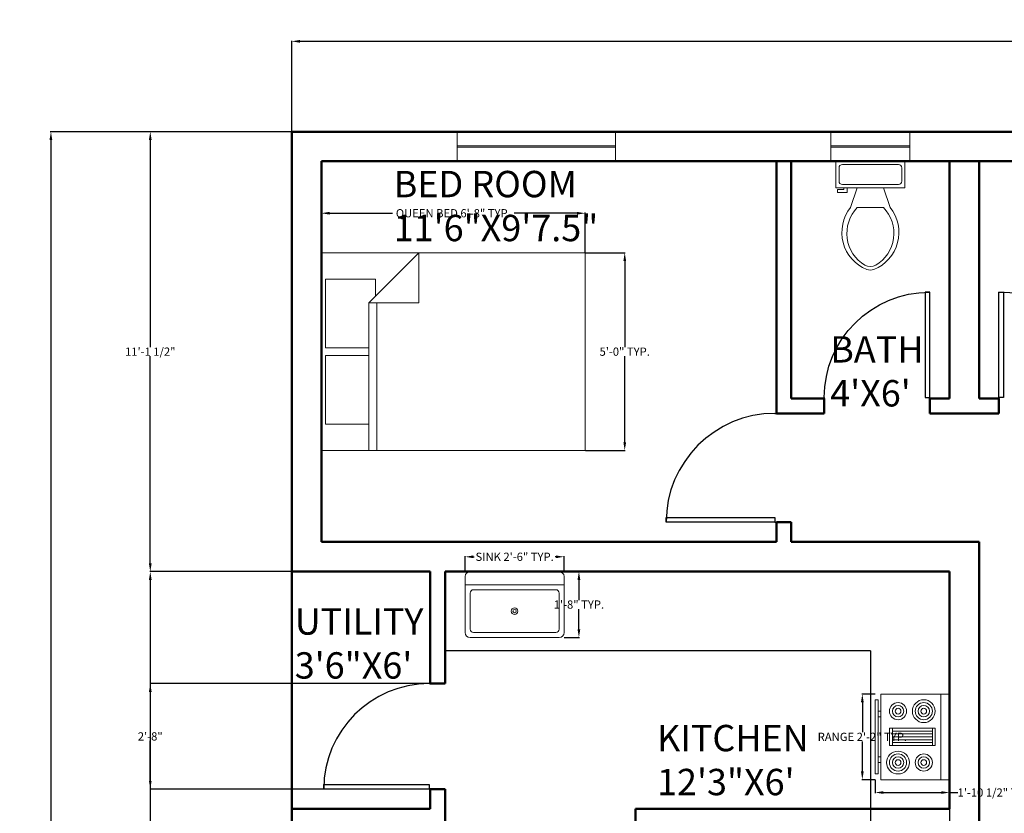
# Model space of a CAD drawing. Units: inches. Extents: x -46 to 565, y -56 to 809.
# Tile 4 of 6: x -46 to 252, y 557 to 798. Entities that reach past the tile are written whole.
import ezdxf

# ---------------------------------------------------------------- set-up
doc = ezdxf.new("R2010")
doc.units = ezdxf.units.IN
doc.header["$MEASUREMENT"] = 0
for name, color, linetype, lineweight in [('A-ANNO-DIMS', 2, 'Continuous', 18), ('A-AREA-IDEN', 241, 'Continuous', 18), ('A-FLOR-CASE', 8, 'Continuous', 25), ('A-FLOR-FIXT', 131, 'Continuous', 18), ('A-FURN', 131, 'Continuous', 18), ('DOOR', 210, 'Continuous', 25), ('EQUIPMENT', 131, 'Continuous', 18), ('WALL', 10, 'Continuous', 50), ('WINDOW', 170, 'Continuous', 18)]:
    doc.layers.add(name, color=color, linetype=linetype, lineweight=lineweight)
doc.styles.get("Standard").update_dxf_attribs({"font": 'arial.ttf'})
doc.dimstyles.get("Standard").update_dxf_attribs({"dimtxt": 2.5, "dimasz": 2.5, "dimexe": 0.18, "dimexo": 0.0625, "dimgap": 0.09, "dimtad": 0, "dimtih": 1, "dimtoh": 1, "dimzin": 0, "dimdsep": 46, "dimlunit": 3, "dimtxsty": 'Standard', "dimcen": 0.09, "dimadec": 0, "dimazin": 0, "dimtfac": 1, "dimtofl": 0, "dimtmove": 0, "dimatfit": 3, "dimfxl": 1, "dimtolj": 1, "dimtzin": 0, "dimarcsym": 0})

# ---------------------------------------------------------------- blocks, each defined once
blk = doc.blocks.new('*U2')
for p, q in [((0, 0), (0, -6)), ((40, 0), (40, -6))]:
    blk.add_line(p, q)
blk.add_lwpolyline([(0, 0), (0, 40), (1.75, 40), (1.75, 0)], close=True)
blk.add_arc((0, 0), 40, 0, 90)
blk = doc.blocks.new('Sink-single - 30 in top')
blk.add_line((-15, -3.999996), (15, -3.999996))
for points in [[(-13.5, 0), (13.5, 0)], [(-15, -18.499996), (-15, -1.5)], [(15, -1.5), (15, -18.499996)], [(-12.5, -5.499996), (12.5, -5.499996)], [(-13.5, -17.499996), (-13.5, -6.499996)], [(13.5, -6.499996), (13.5, -17.499996)], [(13.5, -19.999996), (-13.5, -19.999996)], [(12.5, -18.499996), (-12.5, -18.499996)]]:
    blk.add_lwpolyline(points)
for radius in [1, 0.5]:
    blk.add_circle((0, -11.999996), radius)
for centre, radius, start, end in [((-13.5, -1.5), 1.5, 90, 180), ((13.5, -1.5), 1.5, 0, 90), ((-12.5, -6.499996), 1, 90, 180), ((12.5, -6.499996), 1, 0, 90), ((-12.5, -17.499996), 1, 180, 270), ((12.5, -17.499996), 1, 270, 0), ((-13.5, -18.499996), 1.5, 180, 270), ((13.5, -18.499996), 1.5, 270, 0)]:
    blk.add_arc(centre, radius, start, end)
blk = doc.blocks.new('Bed - Queen')
for p, q in [((0, -80.00003), (0, 0)), ((0, 0), (59.99999, 0)), ((59.99999, 0), (59.99999, -80.00003)), ((7.99999, -1.2), (28.79998, -1.2)), ((7.99999, -14.4), (7.99999, -1.2)), ((28.79998, -1.2), (28.79998, -14.4)), ((31.19999, -1.2), (51.99999, -1.2)), ((31.19999, -14.4), (31.19999, -1.2)), ((51.99999, -1.2), (51.99999, -16.4)), ((0, -14.4), (44.8, -14.4)), ((59.99999, -29.6), (44.8, -14.4)), ((44.8, -14.4), (44.8, -29.6)), ((44.8, -16.8), (0, -16.8)), ((51.99999, -16.4), (46.79936, -16.4)), ((44.8, -29.6), (59.99999, -29.6)), ((59.99999, -80.00003), (0, -80.00003))]:
    blk.add_line(p, q)
blk = doc.blocks.new('Toilet - top')
for p, q in [((9.5, -6), (9.5, -2)), ((-10, -8.5), (-8, -8.5)), ((-10, -9.5), (-10, -8.5)), ((-8, -8.5), (-8, -8)), ((-7, -8), (-7, -9.5)), ((-4, -8), (-6, -14)), ((4, -8), (6, -14)), ((-7, -9.5), (-10, -9.5)), ((4, -14), (-4, -14))]:
    blk.add_line(p, q)
blk.add_lwpolyline([(10.5, -8), (10.5, 0), (-10.5, 0), (-10.5, -8)], close=True)
for points in [[(-9.5, -2), (-9.5, -6)], [(8.5, -1), (-8.5, -1)], [(-8.5, -7), (8.5, -7)]]:
    blk.add_lwpolyline(points)
for centre, radius, start, end in [((-8.62, -1.88), 0.884, 81.8699, 188.1301), ((8.62, -1.88), 0.884, 351.8699, 98.1301), ((-8.62, -6.12), 0.884, 171.8699, 278.1301), ((8.62, -6.12), 0.884, 261.8699, 8.1301), ((3.52, -21.58), 12.17, 141.4691, 247.9714), ((4.2, -21.82), 11.33, 136.3677, 238.9468), ((-3.52, -21.58), 12.17, 292.0284, 38.5307), ((-4.2, -21.82), 11.33, 301.053, 43.6321), ((0, -27.88), 4, 245.7318, 294.2682), ((0, -29), 4, 254.8605, 285.1395)]:
    blk.add_arc(centre, radius, start, end)
blk = doc.blocks.new('Range-Oven - 30 in top')
for p, q in [((0, -3), (30, -3)), ((12, -6), (18, -6)), ((13, -20), (13, -6)), ((14, -6), (14, -20)), ((15, -20), (15, -6)), ((16, -6), (16, -20)), ((17, -20), (17, -6)), ((18, -20), (12, -20)), ((6, -24), (6, -25)), ((8, -25), (8, -24)), ((22, -25), (22, -24)), ((24, -24), (24, -25))]:
    blk.add_line(p, q)
for points in [[(0, -24), (0, 0), (30, 0), (30, -24)], [(12, -21), (12, -5), (18, -5), (18, -21)], [(2, -26), (2, -25), (28, -25), (28, -26)]]:
    blk.add_lwpolyline(points, close=True)
for centre, radius in [((6, -9), 4), ((6, -9), 3), ((24, -9), 3), ((6, -9), 2), ((6, -9), 1), ((24, -9), 2), ((24, -9), 1), ((6, -18), 3), ((6, -18), 2), ((6, -18), 1), ((24, -18), 4), ((24, -18), 3), ((24, -18), 2), ((24, -18), 1)]:
    blk.add_circle(centre, radius)
blk = doc.blocks.new('*D14')
at = {"layer": 'A-ANNO-DIMS', "color": 0, "lineweight": -2, "transparency": 16777216}
for p, q in [((36.14, 764.26), (36.14, 791.8)), ((38.64, 791.62), (267.37, 791.62)), ((513.64, 791.62), (284.92, 791.62)), ((516.14, 764.26), (516.14, 791.8))]:
    blk.add_line(p, q, dxfattribs=at)
at = {"layer": 'A-ANNO-DIMS', "color": 0, "transparency": 16777216}
for points in [[(38.64, 792.04), (38.64, 791.2), (36.14, 791.62)], [(513.64, 792.04), (513.64, 791.2), (516.14, 791.62)]]:
    blk.add_solid(points, dxfattribs=at)
at = {"layer": 'Defpoints', "color": 0, "transparency": 16777216}
for p in [(516.14, 791.62), (36.14, 764.2), (516.14, 764.2)]:
    blk.add_point(p, dxfattribs=at)
at = {"layer": 'A-ANNO-DIMS', "color": 0, "transparency": 16777216, "insert": (276.14, 791.62), "char_height": 10, "attachment_point": 5}
blk.add_mtext("\\A1;40'", dxfattribs=at)
blk = doc.blocks.new('*D15')
at = {"layer": 'A-ANNO-DIMS', "color": 0, "lineweight": -2, "transparency": 16777216}
for p, q in [((174.08, 764.2), (-37.07, 764.2)), ((-36.89, 761.7), (-36.89, 409.4)), ((-36.89, 46.7), (-36.89, 399)), ((174.08, 44.2), (-37.07, 44.2))]:
    blk.add_line(p, q, dxfattribs=at)
at = {"layer": 'A-ANNO-DIMS', "color": 0, "transparency": 16777216}
for points in [[(-37.31, 761.7), (-36.48, 761.7), (-36.89, 764.2)], [(-37.31, 46.7), (-36.48, 46.7), (-36.89, 44.2)]]:
    blk.add_solid(points, dxfattribs=at)
at = {"layer": 'Defpoints', "color": 0, "transparency": 16777216}
for p in [(-36.89, 764.2), (174.14, 764.2), (174.14, 44.2)]:
    blk.add_point(p, dxfattribs=at)
at = {"layer": 'A-ANNO-DIMS', "color": 0, "transparency": 16777216, "insert": (-36.89, 404.2), "char_height": 10, "attachment_point": 5}
blk.add_mtext("\\A1;60'", dxfattribs=at)
blk = doc.blocks.new('WIN-48IN')
for p, q in [((0, 4.75), (48, 4.75)), ((0, 4.25), (48, 4.25))]:
    blk.add_line(p, q)
blk.add_lwpolyline([(0, 0), (48, 0), (48, 9), (0, 9)], close=True)
blk = doc.blocks.new('WIN-24IN')
for p, q in [((4.25, 24), (4.25, 0)), ((4.75, 24), (4.75, 0))]:
    blk.add_line(p, q)
blk.add_lwpolyline([(0, 24), (0, 0), (9, 0), (9, 24)], close=True)
blk = doc.blocks.new('*D19')
at = {"layer": 'A-ANNO-DIMS', "color": 0, "lineweight": -2, "transparency": 16777216}
for p, q in [((45.14, 727.51), (45.14, 739.63)), ((47.64, 739.45), (66.67, 739.45)), ((122.64, 739.45), (103.62, 739.45)), ((125.14, 727.51), (125.14, 739.63))]:
    blk.add_line(p, q, dxfattribs=at)
at = {"layer": 'A-ANNO-DIMS', "color": 0, "transparency": 16777216}
for points in [[(47.64, 739.87), (47.64, 739.03), (45.14, 739.45)], [(122.64, 739.87), (122.64, 739.03), (125.14, 739.45)]]:
    blk.add_solid(points, dxfattribs=at)
at = {"layer": 'Defpoints', "color": 0, "transparency": 16777216}
for p in [(45.14, 739.45), (45.14, 727.45), (125.14, 727.45)]:
    blk.add_point(p, dxfattribs=at)
at = {"layer": 'A-ANNO-DIMS', "color": 0, "transparency": 16777216, "insert": (85.14, 739.45), "char_height": 2.5, "attachment_point": 5}
blk.add_mtext('\\A1;QUEEN BED 6\'-8" TYP.', dxfattribs=at)
blk = doc.blocks.new('*D20')
at = {"layer": 'A-ANNO-DIMS', "color": 0, "lineweight": -2, "transparency": 16777216}
for p, q in [((125.21, 727.45), (137.32, 727.45)), ((137.14, 724.95), (137.14, 698.82)), ((137.14, 669.95), (137.14, 696.08)), ((125.21, 667.45), (137.32, 667.45))]:
    blk.add_line(p, q, dxfattribs=at)
at = {"layer": 'A-ANNO-DIMS', "color": 0, "transparency": 16777216}
for points in [[(136.73, 724.95), (137.56, 724.95), (137.14, 727.45)], [(136.73, 669.95), (137.56, 669.95), (137.14, 667.45)]]:
    blk.add_solid(points, dxfattribs=at)
at = {"layer": 'Defpoints', "color": 0, "transparency": 16777216}
for p in [(125.14, 727.45), (137.14, 727.45), (125.14, 667.45)]:
    blk.add_point(p, dxfattribs=at)
at = {"layer": 'A-ANNO-DIMS', "color": 0, "transparency": 16777216, "insert": (137.14, 697.45), "char_height": 2.5, "attachment_point": 5}
blk.add_mtext('\\A1;5\'-0" TYP.', dxfattribs=at)
blk = doc.blocks.new('*D31')
at = {"layer": 'A-ANNO-DIMS', "color": 0, "lineweight": -2, "transparency": 16777216}
for p, q in [((88.75, 630.76), (88.75, 635.38)), ((91.25, 635.2), (91.48, 635.2)), ((116.25, 635.2), (116.01, 635.2)), ((118.75, 630.76), (118.75, 635.38))]:
    blk.add_line(p, q, dxfattribs=at)
at = {"layer": 'A-ANNO-DIMS', "color": 0, "transparency": 16777216}
for points in [[(91.25, 635.62), (91.25, 634.78), (88.75, 635.2)], [(116.25, 635.62), (116.25, 634.78), (118.75, 635.2)]]:
    blk.add_solid(points, dxfattribs=at)
at = {"layer": 'Defpoints', "color": 0, "transparency": 16777216}
for p in [(88.75, 635.2), (88.75, 630.7), (118.75, 630.7)]:
    blk.add_point(p, dxfattribs=at)
at = {"layer": 'A-ANNO-DIMS', "color": 0, "transparency": 16777216, "insert": (103.75, 635.2), "char_height": 2.5, "attachment_point": 5}
blk.add_mtext('\\A1;SINK 2\'-6" TYP.', dxfattribs=at)
blk = doc.blocks.new('*D32')
at = {"layer": 'A-ANNO-DIMS', "color": 0, "lineweight": -2, "transparency": 16777216}
for p, q in [((118.81, 630.7), (123.43, 630.7)), ((123.25, 628.2), (123.25, 622.07)), ((123.25, 613.2), (123.25, 619.33)), ((118.81, 610.7), (123.43, 610.7))]:
    blk.add_line(p, q, dxfattribs=at)
at = {"layer": 'A-ANNO-DIMS', "color": 0, "transparency": 16777216}
for points in [[(122.83, 628.2), (123.67, 628.2), (123.25, 630.7)], [(122.83, 613.2), (123.67, 613.2), (123.25, 610.7)]]:
    blk.add_solid(points, dxfattribs=at)
at = {"layer": 'Defpoints', "color": 0, "transparency": 16777216}
for p in [(118.75, 630.7), (123.25, 630.7), (118.75, 610.7)]:
    blk.add_point(p, dxfattribs=at)
at = {"layer": 'A-ANNO-DIMS', "color": 0, "transparency": 16777216, "insert": (123.25, 620.7), "char_height": 2.5, "attachment_point": 5}
blk.add_mtext('\\A1;1\'-8" TYP.', dxfattribs=at)
blk = doc.blocks.new('*D35')
at = {"layer": 'A-ANNO-DIMS', "color": 0, "lineweight": -2, "transparency": 16777216}
for p, q in [((213.05, 593.56), (209.03, 593.56)), ((209.21, 591.06), (209.21, 581.94)), ((209.21, 570.06), (209.21, 579.18)), ((213.05, 567.56), (209.03, 567.56))]:
    blk.add_line(p, q, dxfattribs=at)
at = {"layer": 'A-ANNO-DIMS', "color": 0, "transparency": 16777216}
for points in [[(208.79, 591.06), (209.63, 591.06), (209.21, 593.56)], [(208.79, 570.06), (209.63, 570.06), (209.21, 567.56)]]:
    blk.add_solid(points, dxfattribs=at)
at = {"layer": 'Defpoints', "color": 0, "transparency": 16777216}
for p in [(213.11, 593.56), (209.21, 567.56), (213.11, 567.56)]:
    blk.add_point(p, dxfattribs=at)
at = {"layer": 'A-ANNO-DIMS', "color": 0, "transparency": 16777216, "insert": (209.21, 580.56), "char_height": 2.5, "attachment_point": 5}
blk.add_mtext('\\A1;RANGE 2\'-2" TYP.', dxfattribs=at)
blk = doc.blocks.new('*D36')
at = {"layer": 'A-ANNO-DIMS', "color": 0, "lineweight": -2, "transparency": 16777216}
for p, q in [((213.11, 567.5), (213.11, 563.48)), ((235.64, 567.5), (235.64, 563.48)), ((215.61, 563.66), (233.14, 563.66)), ((235.64, 563.66), (238.14, 563.66))]:
    blk.add_line(p, q, dxfattribs=at)
at = {"layer": 'A-ANNO-DIMS', "color": 0, "transparency": 16777216}
for points in [[(215.61, 564.08), (215.61, 563.24), (213.11, 563.66)], [(233.14, 564.08), (233.14, 563.24), (235.64, 563.66)]]:
    blk.add_solid(points, dxfattribs=at)
at = {"layer": 'Defpoints', "color": 0, "transparency": 16777216}
for p in [(213.11, 567.56), (235.64, 567.56), (235.64, 563.66)]:
    blk.add_point(p, dxfattribs=at)
at = {"layer": 'A-ANNO-DIMS', "color": 0, "transparency": 16777216, "insert": (249.62, 563.66), "char_height": 2.5, "attachment_point": 5}
blk.add_mtext('\\A1;1\'-10 1/2" TYP.', dxfattribs=at)
blk = doc.blocks.new('*D46')
at = {"layer": 'A-ANNO-DIMS', "color": 0, "lineweight": -2, "transparency": 16777216}
for p, q in [((36.08, 630.7), (-6.94, 630.7)), ((-6.76, 628.2), (-6.76, 464.54)), ((-6.76, 298.2), (-6.76, 461.85)), ((45.08, 295.7), (-6.94, 295.7))]:
    blk.add_line(p, q, dxfattribs=at)
at = {"layer": 'A-ANNO-DIMS', "color": 0, "transparency": 16777216}
for points in [[(-7.17, 628.2), (-6.34, 628.2), (-6.76, 630.7)], [(-7.17, 298.2), (-6.34, 298.2), (-6.76, 295.7)]]:
    blk.add_solid(points, dxfattribs=at)
at = {"layer": 'Defpoints', "color": 0, "transparency": 16777216}
for p in [(-6.76, 630.7), (36.14, 630.7), (45.14, 295.7)]:
    blk.add_point(p, dxfattribs=at)
at = {"layer": 'A-ANNO-DIMS', "color": 0, "transparency": 16777216, "insert": (-6.76, 463.2), "char_height": 2.5, "attachment_point": 5}
blk.add_mtext('\\A1;27\'-11"', dxfattribs=at)
blk = doc.blocks.new('*D47')
at = {"layer": 'A-ANNO-DIMS', "color": 0, "lineweight": -2, "transparency": 16777216}
for p, q in [((36.08, 764.2), (-6.94, 764.2)), ((-6.76, 761.7), (-6.76, 698.83)), ((-6.76, 633.2), (-6.76, 696.07)), ((36.08, 630.7), (-6.94, 630.7))]:
    blk.add_line(p, q, dxfattribs=at)
at = {"layer": 'A-ANNO-DIMS', "color": 0, "transparency": 16777216}
for points in [[(-7.17, 761.7), (-6.34, 761.7), (-6.76, 764.2)], [(-7.17, 633.2), (-6.34, 633.2), (-6.76, 630.7)]]:
    blk.add_solid(points, dxfattribs=at)
at = {"layer": 'Defpoints', "color": 0, "transparency": 16777216}
for p in [(-6.76, 764.2), (36.14, 764.2), (36.14, 630.7)]:
    blk.add_point(p, dxfattribs=at)
at = {"layer": 'A-ANNO-DIMS', "color": 0, "transparency": 16777216, "insert": (-6.76, 697.45), "char_height": 2.5, "attachment_point": 5}
blk.add_mtext('\\A1;11\'-1 1/2"', dxfattribs=at)
blk = doc.blocks.new('*D50')
at = {"layer": 'A-ANNO-DIMS', "color": 0, "lineweight": -2, "transparency": 16777216}
for p, q in [((211.64, 558.64), (211.64, 0.22)), ((235.64, 558.64), (235.64, 0.22)), ((214.14, 0.4), (220.21, 0.4)), ((233.14, 0.4), (227.08, 0.4))]:
    blk.add_line(p, q, dxfattribs=at)
at = {"layer": 'A-ANNO-DIMS', "color": 0, "transparency": 16777216}
for points in [[(214.14, 0.82), (214.14, -0.02), (211.64, 0.4)], [(233.14, 0.82), (233.14, -0.02), (235.64, 0.4)]]:
    blk.add_solid(points, dxfattribs=at)
at = {"layer": 'Defpoints', "color": 0, "transparency": 16777216}
for p in [(211.64, 558.7), (235.64, 558.7), (235.64, 0.4)]:
    blk.add_point(p, dxfattribs=at)
at = {"layer": 'A-ANNO-DIMS', "color": 0, "transparency": 16777216, "insert": (223.64, 0.4), "char_height": 2.5, "attachment_point": 5}
blk.add_mtext('\\A1;2\'-0"', dxfattribs=at)
blk = doc.blocks.new('*D52')
at = {"layer": 'A-ANNO-DIMS', "color": 0, "lineweight": -2, "transparency": 16777216}
for p, q in [((78.08, 596.7), (-6.94, 596.7)), ((-6.76, 594.2), (-6.76, 582.07)), ((-6.76, 567.2), (-6.76, 579.33)), ((78.08, 564.7), (-6.94, 564.7))]:
    blk.add_line(p, q, dxfattribs=at)
at = {"layer": 'A-ANNO-DIMS', "color": 0, "transparency": 16777216}
for points in [[(-7.17, 594.2), (-6.34, 594.2), (-6.76, 596.7)], [(-7.17, 567.2), (-6.34, 567.2), (-6.76, 564.7)]]:
    blk.add_solid(points, dxfattribs=at)
at = {"layer": 'Defpoints', "color": 0, "transparency": 16777216}
for p in [(-6.76, 596.7), (78.14, 596.7), (78.14, 564.7)]:
    blk.add_point(p, dxfattribs=at)
at = {"layer": 'A-ANNO-DIMS', "color": 0, "transparency": 16777216, "insert": (-6.76, 580.7), "char_height": 2.5, "attachment_point": 5}
blk.add_mtext('\\A1;2\'-8"', dxfattribs=at)

msp = doc.modelspace()

# ---------------------------------------------------------------- linework, layer by layer
at = {"layer": 'A-FLOR-CASE'}
for q in [(82.643, 606.7), (211.643, 558.7)]:
    msp.add_line((211.643, 606.7), q, dxfattribs=at)
at = {"layer": 'WALL'}
for p, q in [((516.143, 764.2), (36.143, 764.2)), ((36.143, 764.2), (36.143, 630.7)), ((45.143, 755.2), (45.143, 639.7)), ((187.643, 755.2), (45.143, 755.2)), ((183.143, 755.2), (183.143, 678.7)), ((187.643, 755.2), (187.643, 683.2)), ((235.643, 755.2), (187.643, 755.2)), ((235.643, 755.2), (235.643, 683.2)), ((244.643, 755.2), (235.643, 755.2)), ((244.643, 755.2), (244.643, 683.2)), ((292.643, 755.2), (244.643, 755.2)), ((197.643, 683.2), (187.643, 683.2)), ((197.643, 683.2), (197.643, 678.7)), ((235.643, 683.2), (229.643, 683.2)), ((229.643, 683.2), (229.643, 678.7)), ((250.643, 683.2), (244.643, 683.2)), ((250.643, 683.2), (250.643, 678.7)), ((187.643, 678.7), (183.143, 678.7)), ((197.643, 678.7), (187.643, 678.7)), ((235.643, 678.7), (229.643, 678.7)), ((235.643, 678.7), (244.643, 678.7)), ((250.643, 678.7), (244.643, 678.7)), ((183.143, 645.7), (187.643, 645.7)), ((183.143, 645.7), (183.143, 639.7)), ((187.643, 645.7), (187.643, 639.7)), ((183.143, 639.7), (45.143, 639.7)), ((235.643, 639.7), (187.643, 639.7)), ((235.643, 639.7), (244.643, 639.7)), ((244.643, 639.7), (244.643, 635.2)), ((244.643, 635.2), (244.643, 462.2)), ((36.143, 630.7), (36.143, 558.7)), ((78.143, 630.7), (36.143, 630.7)), ((78.143, 630.7), (78.143, 596.7)), ((82.643, 630.7), (82.643, 596.7)), ((235.643, 630.7), (82.643, 630.7)), ((235.643, 630.7), (235.643, 558.7)), ((78.143, 596.7), (82.643, 596.7)), ((78.143, 564.7), (82.643, 564.7)), ((78.143, 564.7), (78.143, 558.7)), ((82.643, 564.7), (82.643, 558.7)), ((36.143, 558.7), (36.143, 402.7)), ((78.143, 558.7), (36.143, 558.7)), ((82.643, 558.7), (82.643, 554.2)), ((235.643, 558.7), (140.418, 558.7)), ((140.418, 558.7), (140.418, 554.2))]:
    msp.add_line(p, q, dxfattribs=at)

# ---------------------------------------------------------------- block references
at = {"layer": 'A-FLOR-FIXT'}
msp.add_blockref('Toilet - top', (211.643, 755.2), dxfattribs=at)
at = {"layer": 'A-FLOR-FIXT', "xscale": -1}
msp.add_blockref('Sink-single - 30 in top', (103.749, 630.7), dxfattribs=at)
at = {"layer": 'A-FURN', "rotation": 90}
msp.add_blockref('Bed - Queen', (45.143, 667.45), dxfattribs=at)
at = {"layer": 'DOOR', "yscale": 0.8, "zscale": 0.8}
for p, xscale in [((229.643, 683.5), -0.8), ((250.643, 683.5), 0.8)]:
    msp.add_blockref('*U2', p, dxfattribs=dict(at, xscale=xscale))
at = {"layer": 'DOOR', "rotation": 90}
for p, xscale, yscale, zscale in [((182.693, 645.7), 0.825, 0.825, 0.825), ((77.843, 564.7), 0.8, 0.8, 0.8)]:
    msp.add_blockref('*U2', p, dxfattribs=dict(at, xscale=xscale, yscale=yscale, zscale=zscale))
at = {"layer": 'EQUIPMENT', "xscale": 0.8666666666666667, "yscale": 0.8666666666666667, "zscale": 0.8666666666666667, "rotation": 270}
msp.add_blockref('Range-Oven - 30 in top', (235.643, 593.559), dxfattribs=at)
at = {"layer": 'WINDOW'}
msp.add_blockref('WIN-48IN', (86.359, 755.2), dxfattribs=at)
at = {"layer": 'WINDOW', "rotation": 270.0000000000004}
msp.add_blockref('WIN-24IN', (199.643, 764.2), dxfattribs=at)

# ---------------------------------------------------------------- texts
at = {"layer": 'A-AREA-IDEN', "char_height": 8, "attachment_point": 1}
for s, insert in [('BED ROOM\\P11\'6"X9\'7.5" ', (67.071, 752.301)), ("BATH\\P4'X6'", (199.464, 702.146)), ('UTILITY\\P3\'6"X6\' ', (37.054, 619.569)), ('KITCHEN\\P12\'3"X6\' ', (146.933, 584.185))]:
    msp.add_mtext_dynamic_manual_height_columns(s, width=70.77133, gutter_width=1, heights=[0], dxfattribs=dict(at, insert=insert))

# ---------------------------------------------------------------- dimensions: what is measured, and where the dimension line sits
at = {"layer": 'A-ANNO-DIMS'}
for p1, p2, distance, picture, middle in [((36.143, 764.2), (516.143, 764.2), 27.422, '*D14', (276.143, 791.621)), ((174.143, 44.2), (174.143, 764.2), 211.037, '*D15', (-36.894, 404.2))]:
    dim = msp.add_aligned_dim(p1=p1, p2=p2, distance=distance, dimstyle='Standard', override={"dimtxt": 10, "dimclrd": 0, "dimclre": 0, "dimclrt": 0}, dxfattribs=at)
    dim.commit()
    dim.dimension.update_dxf_attribs({"geometry": picture, "text_midpoint": middle})
for base, p1, p2, picture, middle in [((-6.757, 764.2), (36.143, 630.7), (36.143, 764.2), '*D47', (-6.757, 697.45)), ((-6.757, 630.7), (45.143, 295.7), (36.143, 630.7), '*D46', (-6.757, 463.2)), ((-6.757, 596.7), (78.143, 564.7), (78.143, 596.7), '*D52', (-6.757, 580.7))]:
    dim = msp.add_linear_dim(base=base, p1=p1, p2=p2, angle=90, dimstyle='Standard', override={"dimdec": 1, "dimlfac": 1, "dimrnd": 0, "dimzin": 1, "dimdsep": 46, "dimlunit": 4, "dimfrac": 2}, dxfattribs=at)
    dim.commit()
    dim.dimension.update_dxf_attribs({"geometry": picture, "text_midpoint": middle})
for base, p1, p2, angle, text, picture, middle in [((45.143, 739.45), (125.143, 727.45), (45.143, 727.45), 180, 'QUEEN BED <> TYP.', '*D19', (85.143, 739.45)), ((137.143, 727.45), (125.143, 667.45), (125.143, 727.45), 90, '<> TYP.', '*D20', (137.143, 697.45)), ((88.749, 635.2), (118.749, 630.7), (88.749, 630.7), 180, 'SINK <> TYP.', '*D31', (103.749, 635.2)), ((123.249, 630.7), (118.749, 610.7), (118.749, 630.7), 90, '<> TYP.', '*D32', (123.249, 620.7)), ((209.21, 567.559), (213.11, 593.559), (213.11, 567.559), 270, 'RANGE <> TYP.', '*D35', (209.21, 580.559))]:
    dim = msp.add_linear_dim(base=base, p1=p1, p2=p2, angle=angle, text=text, dimstyle='Standard', override={"dimdec": 1, "dimlfac": 1, "dimrnd": 0, "dimzin": 1, "dimdsep": 46, "dimlunit": 4, "dimfrac": 2}, dxfattribs=at)
    dim.commit()
    dim.dimension.update_dxf_attribs({"geometry": picture, "text_midpoint": middle})
dim = msp.add_linear_dim(base=(235.643, 563.659), p1=(213.11, 567.559), p2=(235.643, 567.559), text='<> TYP.', dimstyle='Standard', override={"dimdec": 1, "dimlfac": 1, "dimrnd": 0, "dimzin": 1, "dimdsep": 46, "dimlunit": 4, "dimfrac": 2}, dxfattribs=at)
dim.commit()
dim.dimension.update_dxf_attribs({"geometry": '*D36', "text_midpoint": (249.618, 563.659)})
dim = msp.add_linear_dim(base=(235.643, 0.4), p1=(211.643, 558.7), p2=(235.643, 558.7), dimstyle='Standard', override={"dimdec": 1, "dimlfac": 1, "dimrnd": 0, "dimzin": 1, "dimdsep": 46, "dimlunit": 4, "dimfrac": 2}, dxfattribs=at)
dim.commit()
dim.dimension.update_dxf_attribs({"geometry": '*D50', "text_midpoint": (223.643, 0.4)})

doc.saveas('drawing.dxf')
